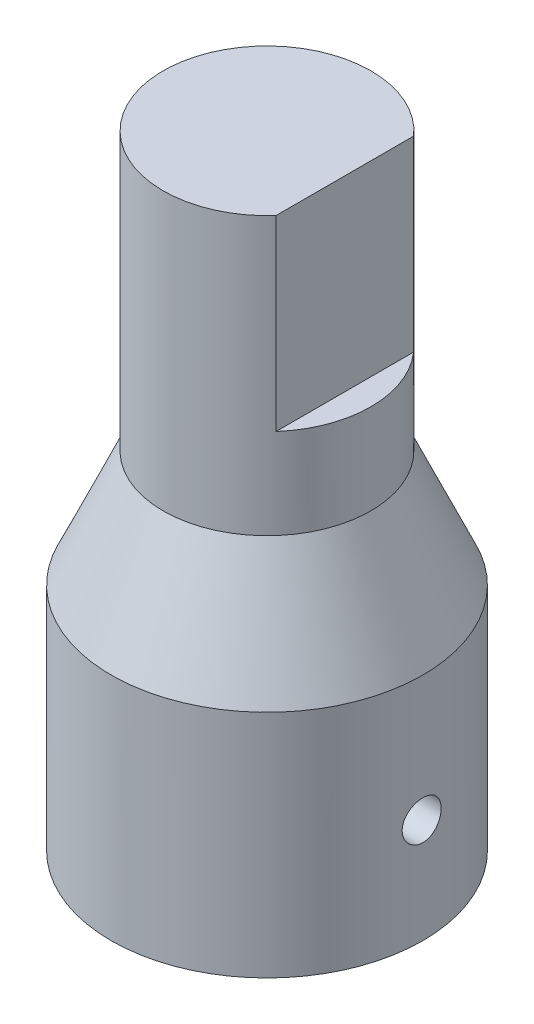
ISO-10303-21;
HEADER;
FILE_DESCRIPTION(('STEP AP214'),'2;1');
FILE_NAME('part.step','',(''),(''),'','','');
FILE_SCHEMA(('AUTOMOTIVE_DESIGN { 1 0 10303 214 1 1 1 1 }'));
ENDSEC;
DATA;
#1=APPLICATION_CONTEXT('core data for automotive mechanical design processes');
#2=APPLICATION_PROTOCOL_DEFINITION('international standard','automotive_design',2000,#1);
#3=PRODUCT_CONTEXT('',#1,'mechanical');
#4=PRODUCT('Part','Part','',(#3));
#5=PRODUCT_RELATED_PRODUCT_CATEGORY('part','',(#4));
#6=PRODUCT_DEFINITION_FORMATION('','',#4);
#7=PRODUCT_DEFINITION_CONTEXT('part definition',#1,'design');
#8=PRODUCT_DEFINITION('design','',#6,#7);
#9=PRODUCT_DEFINITION_SHAPE('','',#8);
#10=(LENGTH_UNIT() NAMED_UNIT(*) SI_UNIT(.MILLI.,.METRE.));
#11=(NAMED_UNIT(*) PLANE_ANGLE_UNIT() SI_UNIT($,.RADIAN.));
#12=(NAMED_UNIT(*) SI_UNIT($,.STERADIAN.) SOLID_ANGLE_UNIT());
#13=UNCERTAINTY_MEASURE_WITH_UNIT(LENGTH_MEASURE(1.E-05),#10,'distance_accuracy_value','');
#14=(GEOMETRIC_REPRESENTATION_CONTEXT(3) GLOBAL_UNCERTAINTY_ASSIGNED_CONTEXT((#13)) GLOBAL_UNIT_ASSIGNED_CONTEXT((#10,
#11,#12)) REPRESENTATION_CONTEXT('',''));
#15=CARTESIAN_POINT('',(0.,0.,0.));
#16=DIRECTION('',(0.,0.,1.));
#17=DIRECTION('',(1.,0.,0.));
#18=AXIS2_PLACEMENT_3D('',#15,#16,#17);
#19=CARTESIAN_POINT('',(0.,14.06,0.));
#20=DIRECTION('',(0.,-1.,0.));
#21=DIRECTION('',(0.,0.,-1.));
#22=AXIS2_PLACEMENT_3D('',#19,#20,#21);
#23=CYLINDRICAL_SURFACE('',#22,9.525);
#24=CARTESIAN_POINT('',(0.,14.06,0.));
#25=DIRECTION('',(0.,-1.,0.));
#26=DIRECTION('',(0.,0.,-1.));
#27=AXIS2_PLACEMENT_3D('',#24,#25,#26);
#28=CIRCLE('',#27,9.525);
#29=CARTESIAN_POINT('',(0.,14.06,-9.525));
#30=VERTEX_POINT('',#29);
#31=EDGE_CURVE('E79',#30,#30,#28,.F.);
#32=ORIENTED_EDGE('',*,*,#31,.F.);
#33=EDGE_LOOP('',(#32));
#34=FACE_BOUND('',#33,.T.);
#35=CARTESIAN_POINT('',(0.,0.,0.));
#36=DIRECTION('',(0.,1.,0.));
#37=DIRECTION('',(0.,0.,1.));
#38=AXIS2_PLACEMENT_3D('',#35,#36,#37);
#39=CIRCLE('',#38,9.525);
#40=CARTESIAN_POINT('',(0.,0.,9.525));
#41=VERTEX_POINT('',#40);
#42=EDGE_CURVE('E91',#41,#41,#39,.T.);
#43=ORIENTED_EDGE('',*,*,#42,.T.);
#44=EDGE_LOOP('',(#43));
#45=FACE_BOUND('',#44,.T.);
#46=CARTESIAN_POINT('',(9.45037168581215,6.38,1.19));
#47=CARTESIAN_POINT('',(9.45037264153151,6.31343763360096,1.18999716991653));
#48=CARTESIAN_POINT('',(9.45108251308956,6.24683365884784,1.1843964303129));
#49=CARTESIAN_POINT('',(9.45384422599999,6.11547928977974,1.16214251532668));
#50=CARTESIAN_POINT('',(9.45589746984964,6.05073090654836,1.14547778873659));
#51=CARTESIAN_POINT('',(9.46110981514661,5.92500853678741,1.10159483656561));
#52=CARTESIAN_POINT('',(9.46426816613176,5.86403202182239,1.07438377150283));
#53=CARTESIAN_POINT('',(9.47133395466148,5.7475222134488,1.01019588043544));
#54=CARTESIAN_POINT('',(9.47524126405582,5.691987991292,0.973220724703552));
#55=CARTESIAN_POINT('',(9.48338917829167,5.58761734378629,0.890332801063359));
#56=CARTESIAN_POINT('',(9.48763134988199,5.53881574535426,0.844376329040483));
#57=CARTESIAN_POINT('',(9.49595691130435,5.44959647319169,0.744924376498652));
#58=CARTESIAN_POINT('',(9.50004029323059,5.40917921646723,0.691428521220839));
#59=CARTESIAN_POINT('',(9.5076042146436,5.33775104258135,0.578197512107269));
#60=CARTESIAN_POINT('',(9.51108271819785,5.30677163849966,0.518442331675223));
#61=CARTESIAN_POINT('',(9.51702773167735,5.25530040739616,0.394526840092954));
#62=CARTESIAN_POINT('',(9.51949427912391,5.23480819152343,0.330366692373087));
#63=CARTESIAN_POINT('',(9.52312643380533,5.20499707510872,0.199818674007887));
#64=CARTESIAN_POINT('',(9.52429877975999,5.19562027914244,0.133444214479628));
#65=CARTESIAN_POINT('',(9.52523345022345,5.18812675008786,5.4171031885184E-05));
#66=CARTESIAN_POINT('',(9.52499583014668,5.19000957447439,-0.0669613875877963));
#67=CARTESIAN_POINT('',(9.52314279467513,5.20493543907906,-0.199337403060523));
#68=CARTESIAN_POINT('',(9.52153506646859,5.2179162139632,-0.264705003295682));
#69=CARTESIAN_POINT('',(9.51713109983186,5.2545721705004,-0.392326661691793));
#70=CARTESIAN_POINT('',(9.5143348388273,5.27824755528178,-0.454580660689544));
#71=CARTESIAN_POINT('',(9.50785476589063,5.33568689520442,-0.57440072392236));
#72=CARTESIAN_POINT('',(9.5041685883766,5.36947779791912,-0.631953736900307));
#73=CARTESIAN_POINT('',(9.49632108787332,5.44616937011639,-0.740595739392311));
#74=CARTESIAN_POINT('',(9.49215974311959,5.48907045695765,-0.791684432589693));
#75=CARTESIAN_POINT('',(9.4837940809287,5.58311333196171,-0.886313374417254));
#76=CARTESIAN_POINT('',(9.47958966407611,5.63430938396301,-0.929799704260077));
#77=CARTESIAN_POINT('',(9.47163976542179,5.74330250640203,-1.00757044992837));
#78=CARTESIAN_POINT('',(9.46789428505592,5.80109959749108,-1.04185483696445));
#79=CARTESIAN_POINT('',(9.461286366945,5.92170218000654,-1.10025156744196));
#80=CARTESIAN_POINT('',(9.45842430411225,5.98450978364658,-1.12435959374305));
#81=CARTESIAN_POINT('',(9.45391457914727,6.11332556338726,-1.16167145862918));
#82=CARTESIAN_POINT('',(9.45226685855337,6.17933358524813,-1.17487582214934));
#83=CARTESIAN_POINT('',(9.4503830576482,6.31220027581877,-1.18993413525669));
#84=CARTESIAN_POINT('',(9.45013754054481,6.37905021610411,-1.19186396418473));
#85=CARTESIAN_POINT('',(9.45106098640868,6.51212045912965,-1.18451863421254));
#86=CARTESIAN_POINT('',(9.45222991925946,6.57834077524554,-1.17524371388379));
#87=CARTESIAN_POINT('',(9.45584194377805,6.70804463948868,-1.14581605336035));
#88=CARTESIAN_POINT('',(9.45828073101195,6.77153665354108,-1.125700053228));
#89=CARTESIAN_POINT('',(9.46415418223574,6.89424645557599,-1.07519907196292));
#90=CARTESIAN_POINT('',(9.46758888117965,6.95346409344744,-1.04481373039573));
#91=CARTESIAN_POINT('',(9.47508975436793,7.06628748014224,-0.974450020430184));
#92=CARTESIAN_POINT('',(9.47915916429753,7.1198619761186,-0.934421890790981));
#93=CARTESIAN_POINT('',(9.48746077568779,7.21955941966134,-0.845979202945391));
#94=CARTESIAN_POINT('',(9.49169298346884,7.26568207755892,-0.797564318879548));
#95=CARTESIAN_POINT('',(9.4998723107226,7.34943313065488,-0.693390980417168));
#96=CARTESIAN_POINT('',(9.5038176697801,7.38701166665858,-0.637592283310463));
#97=CARTESIAN_POINT('',(9.51095243606812,7.45226276847941,-0.520430956263431));
#98=CARTESIAN_POINT('',(9.51414185852176,7.4799355337856,-0.459068438402256));
#99=CARTESIAN_POINT('',(9.51939757374525,7.52450722689759,-0.332687033687352));
#100=CARTESIAN_POINT('',(9.52146686860327,7.54143497401439,-0.267678440724219));
#101=CARTESIAN_POINT('',(9.52426163977849,7.56412986511567,-0.135714153998385));
#102=CARTESIAN_POINT('',(9.52498717662689,7.56989751182084,-0.0687585480792384));
#103=CARTESIAN_POINT('',(9.52501239888289,7.57009909151163,0.0647122895703891));
#104=CARTESIAN_POINT('',(9.52432175662993,7.56460990732446,0.131227416461207));
#105=CARTESIAN_POINT('',(9.52161144912067,7.54261647241155,0.26238193590744));
#106=CARTESIAN_POINT('',(9.51959178478192,7.52611222929047,0.327021329757808));
#107=CARTESIAN_POINT('',(9.51444936789292,7.48258130341164,0.452579463158118));
#108=CARTESIAN_POINT('',(9.51132700095355,7.45555829868751,0.513499494631467));
#109=CARTESIAN_POINT('',(9.50432492428026,7.39176490093249,0.629952236022893));
#110=CARTESIAN_POINT('',(9.50044520558124,7.35499439251425,0.685484882156463));
#111=CARTESIAN_POINT('',(9.4923298874484,7.27246531130851,0.789979263186505));
#112=CARTESIAN_POINT('',(9.48809212661981,7.2266495327557,0.838895652055997));
#113=CARTESIAN_POINT('',(9.47975569136095,7.1274492229981,0.928376018315304));
#114=CARTESIAN_POINT('',(9.47565705011555,7.07406290146226,0.968938014423616));
#115=CARTESIAN_POINT('',(9.46804605795317,6.96100081172117,1.04069195281877));
#116=CARTESIAN_POINT('',(9.46453602974224,6.90130157540942,1.07184714494874));
#117=CARTESIAN_POINT('',(9.45852691404486,6.77750807150617,1.12364570369548));
#118=CARTESIAN_POINT('',(9.4560267275397,6.71341867112672,1.14430050434002));
#119=CARTESIAN_POINT('',(9.45292749587681,6.60416460922818,1.16956651409533));
#120=CARTESIAN_POINT('',(9.45197383987563,6.55968909404729,1.17721805327143));
#121=CARTESIAN_POINT('',(9.45069561356315,6.47014874568561,1.18743573539382));
#122=CARTESIAN_POINT('',(9.45037103848582,6.42508391697216,1.19000191686767));
#123=CARTESIAN_POINT('',(9.45037168581215,6.38,1.19));
#124=B_SPLINE_CURVE_WITH_KNOTS('',3,(#46,#47,#48,#49,#50,#51,#52,#53,#54,#55,#56,#57,#58,#59,
#60,#61,#62,#63,#64,#65,#66,#67,#68,#69,#70,#71,#72,#73,#74,#75,#76,#77,#78,#79,#80,#81,#82,#83,
#84,#85,#86,#87,#88,#89,#90,#91,#92,#93,#94,#95,#96,#97,#98,#99,#100,#101,#102,#103,#104,#105,
#106,#107,#108,#109,#110,#111,#112,#113,#114,#115,#116,#117,#118,#119,#120,#121,#122,#123),
.UNSPECIFIED.,.T.,.F.,(4,2,2,2,2,2,2,2,2,2,2,2,2,2,2,2,2,2,2,2,2,2,2,2,2,2,2,2,2,2,2,2,2,2,2,2,
2,2,4),(0.,0.199522399972923,0.399253436900873,0.598849101788066,0.798410645373971,
0.998968609282526,1.19953654581048,1.40076702034379,1.60199003297955,1.80216029108681,
2.00232268216225,2.20136937178266,2.40041984215972,2.60000537137378,2.79960004603763,
3.00055746048545,3.20151550364546,3.40255871421423,3.60359224539375,3.80327121734763,
4.00294593781248,4.20194818383015,4.4009574151758,4.60101649566635,4.80108335100855,
5.00228933136802,5.20349125947837,5.40415123610588,5.60480217354306,5.80408725360614,
6.00337219608515,6.20258751827357,6.40180519880469,6.6023256823584,6.80289366562246,
7.00423537300967,7.20535736435751,7.34049858531238,7.47563878241023),.UNSPECIFIED.);
#125=CARTESIAN_POINT('',(9.45037168581215,6.38,1.19));
#126=VERTEX_POINT('',#125);
#127=EDGE_CURVE('E137',#126,#126,#124,.T.);
#128=ORIENTED_EDGE('',*,*,#127,.F.);
#129=EDGE_LOOP('',(#128));
#130=FACE_BOUND('',#129,.T.);
#131=ADVANCED_FACE('F43',(#34,#45,#130),#23,.T.);
#132=CARTESIAN_POINT('',(0.,14.06,0.));
#133=DIRECTION('',(0.,-1.,0.));
#134=DIRECTION('',(0.,0.,-1.));
#135=AXIS2_PLACEMENT_3D('',#132,#133,#134);
#136=CYLINDRICAL_SURFACE('',#135,6.35);
#137=CARTESIAN_POINT('',(0.,14.06,0.));
#138=DIRECTION('',(0.,-1.,0.));
#139=DIRECTION('',(0.,0.,-1.));
#140=AXIS2_PLACEMENT_3D('',#137,#138,#139);
#141=CIRCLE('',#140,6.35);
#142=CARTESIAN_POINT('',(0.,14.06,-6.35));
#143=VERTEX_POINT('',#142);
#144=EDGE_CURVE('E144',#143,#143,#141,.T.);
#145=ORIENTED_EDGE('',*,*,#144,.F.);
#146=EDGE_LOOP('',(#145));
#147=FACE_BOUND('',#146,.T.);
#148=CARTESIAN_POINT('',(0.,0.,0.));
#149=DIRECTION('',(0.,-1.,0.));
#150=DIRECTION('',(0.,0.,-1.));
#151=AXIS2_PLACEMENT_3D('',#148,#149,#150);
#152=CIRCLE('',#151,6.35);
#153=CARTESIAN_POINT('',(0.,0.,-6.35));
#154=VERTEX_POINT('',#153);
#155=EDGE_CURVE('E142',#154,#154,#152,.T.);
#156=ORIENTED_EDGE('',*,*,#155,.T.);
#157=EDGE_LOOP('',(#156));
#158=FACE_BOUND('',#157,.T.);
#159=CARTESIAN_POINT('',(6.23749949899798,6.38,1.19));
#160=CARTESIAN_POINT('',(6.23750078026261,6.44621005322413,1.18999745972019));
#161=CARTESIAN_POINT('',(6.23856516125152,6.51245307174854,1.18445549061902));
#162=CARTESIAN_POINT('',(6.24270238343881,6.6430712585922,1.16244896292699));
#163=CARTESIAN_POINT('',(6.24577692913486,6.70744479327753,1.14597513460551));
#164=CARTESIAN_POINT('',(6.25357431695067,6.83241517642426,1.10262852836323));
#165=CARTESIAN_POINT('',(6.25829562402851,6.89301548034891,1.07576543235335));
#166=CARTESIAN_POINT('',(6.2688527438643,7.00884538232623,1.01242846911454));
#167=CARTESIAN_POINT('',(6.2746884694542,7.06407539992465,0.97595535348152));
#168=CARTESIAN_POINT('',(6.28689792642734,7.16828773759325,0.893950345694622));
#169=CARTESIAN_POINT('',(6.29327692734904,7.21719359759681,0.848322057689071));
#170=CARTESIAN_POINT('',(6.30580763864063,7.30670319626329,0.749510255370385));
#171=CARTESIAN_POINT('',(6.31195933407418,7.34730639014685,0.696326245676426));
#172=CARTESIAN_POINT('',(6.32339874913363,7.4193510367955,0.583410530974325));
#173=CARTESIAN_POINT('',(6.32867953647516,7.4507204053366,0.523632070986402));
#174=CARTESIAN_POINT('',(6.33772315208374,7.50294252845517,0.399537974600996));
#175=CARTESIAN_POINT('',(6.34148610501512,7.5237961467582,0.335222711334857));
#176=CARTESIAN_POINT('',(6.34703284970264,7.55415839406284,0.204672981861456));
#177=CARTESIAN_POINT('',(6.34883910987182,7.56379591352581,0.138469462402981));
#178=CARTESIAN_POINT('',(6.35034639387622,7.57185398879645,0.0053621812782321));
#179=CARTESIAN_POINT('',(6.35004759679846,7.57027549880209,-0.0615415203367523));
#180=CARTESIAN_POINT('',(6.34739599219528,7.55604522087716,-0.193266108981925));
#181=CARTESIAN_POINT('',(6.34506892879018,7.54353221603618,-0.258102581921304));
#182=CARTESIAN_POINT('',(6.33865113768287,7.50800759901928,-0.38473898180573));
#183=CARTESIAN_POINT('',(6.33456034575559,7.48499560452736,-0.446538798081501));
#184=CARTESIAN_POINT('',(6.32503171329325,7.42899396992299,-0.565750219062392));
#185=CARTESIAN_POINT('',(6.31958641289168,7.39594884288113,-0.623135137199623));
#186=CARTESIAN_POINT('',(6.3079509674285,7.32085985738842,-0.731597201950985));
#187=CARTESIAN_POINT('',(6.30176074672389,7.27881508472967,-0.782673706907869));
#188=CARTESIAN_POINT('',(6.28920920850321,7.18615551631969,-0.877891333959208));
#189=CARTESIAN_POINT('',(6.28284672261843,7.13541930570736,-0.921914229747355));
#190=CARTESIAN_POINT('',(6.27075839278776,7.02722155734565,-1.00084384377462));
#191=CARTESIAN_POINT('',(6.26503255813905,6.96975992140816,-1.03575042889576));
#192=CARTESIAN_POINT('',(6.25486413987407,6.84958578294708,-1.09549021666779));
#193=CARTESIAN_POINT('',(6.25042374700944,6.78686454843463,-1.12030625097985));
#194=CARTESIAN_POINT('',(6.2433625311351,6.65804095956337,-1.15901479823213));
#195=CARTESIAN_POINT('',(6.24074150218919,6.59193898878427,-1.17290854750374));
#196=CARTESIAN_POINT('',(6.23765651246904,6.45929638123639,-1.18920554320072));
#197=CARTESIAN_POINT('',(6.23716066944776,6.39277733272415,-1.19177863887631));
#198=CARTESIAN_POINT('',(6.23829687782516,6.26026005370896,-1.18581657464029));
#199=CARTESIAN_POINT('',(6.23992882410675,6.19426179763987,-1.17728196347184));
#200=CARTESIAN_POINT('',(6.24510703467551,6.06521785772552,-1.14949255723867));
#201=CARTESIAN_POINT('',(6.24863739352759,6.00215230597804,-1.13032679150002));
#202=CARTESIAN_POINT('',(6.25720094453764,5.88012761734596,-1.08191358131688));
#203=CARTESIAN_POINT('',(6.26223424735253,5.82116878322011,-1.05266539451161));
#204=CARTESIAN_POINT('',(6.27330916940283,5.7082828543774,-0.984526619256281));
#205=CARTESIAN_POINT('',(6.27936174687189,5.65442162423767,-0.945528727348812));
#206=CARTESIAN_POINT('',(6.29176241291361,5.5539461255804,-0.859142256605887));
#207=CARTESIAN_POINT('',(6.2981105279895,5.5073325086472,-0.81175292417047));
#208=CARTESIAN_POINT('',(6.31048943918087,5.42204094145246,-0.709170216058338));
#209=CARTESIAN_POINT('',(6.316514868931,5.38347721693516,-0.653881118633038));
#210=CARTESIAN_POINT('',(6.32747922465622,5.31618624816834,-0.537510237310789));
#211=CARTESIAN_POINT('',(6.33241819242796,5.28745862549619,-0.476428676381761));
#212=CARTESIAN_POINT('',(6.34063005728923,5.24082635641034,-0.350522475511806));
#213=CARTESIAN_POINT('',(6.34391157822906,5.22286559572911,-0.285719205908492));
#214=CARTESIAN_POINT('',(6.34847559724797,5.19809780528843,-0.153948610563211));
#215=CARTESIAN_POINT('',(6.34975830543563,5.19128960320511,-0.086981513031147));
#216=CARTESIAN_POINT('',(6.35017600053786,5.18906096960872,0.0461203195725555));
#217=CARTESIAN_POINT('',(6.34934352630838,5.19346801033821,0.112252125580659));
#218=CARTESIAN_POINT('',(6.3456920050971,5.21316692161687,0.242815271554796));
#219=CARTESIAN_POINT('',(6.34287297711735,5.22845868804999,0.30724662778009));
#220=CARTESIAN_POINT('',(6.33556507456714,5.26942030676389,0.432488844623476));
#221=CARTESIAN_POINT('',(6.33107915298483,5.29507181317,0.493305888490748));
#222=CARTESIAN_POINT('',(6.32092309466721,5.35600408370262,0.609798425416549));
#223=CARTESIAN_POINT('',(6.3152528787102,5.39128549205617,0.665473574155821));
#224=CARTESIAN_POINT('',(6.3032515687894,5.47106999737169,0.770961663863636));
#225=CARTESIAN_POINT('',(6.29691218406044,5.51569774504503,0.820679394552785));
#226=CARTESIAN_POINT('',(6.28433937847151,5.61264944961917,0.911980157400864));
#227=CARTESIAN_POINT('',(6.2781059828841,5.66497521414173,0.953561273589892));
#228=CARTESIAN_POINT('',(6.26638797766641,5.77641607881666,1.02776945897011));
#229=CARTESIAN_POINT('',(6.26091082012314,5.8355894524784,1.06031023015317));
#230=CARTESIAN_POINT('',(6.25141509395909,5.95864671949259,1.11493693768154));
#231=CARTESIAN_POINT('',(6.24739514899,6.02252609899368,1.13703274540451));
#232=CARTESIAN_POINT('',(6.2421074557308,6.13549524949637,1.16565023261791));
#233=CARTESIAN_POINT('',(6.24038973096045,6.18392352847998,1.17476575000297));
#234=CARTESIAN_POINT('',(6.23808529163837,6.28156181125071,1.18694149580345));
#235=CARTESIAN_POINT('',(6.23749854635776,6.33077179376219,1.19000188873762));
#236=CARTESIAN_POINT('',(6.23749949899798,6.38,1.19));
#237=B_SPLINE_CURVE_WITH_KNOTS('',3,(#159,#160,#161,#162,#163,#164,#165,#166,#167,#168,#169,
#170,#171,#172,#173,#174,#175,#176,#177,#178,#179,#180,#181,#182,#183,#184,#185,#186,#187,#188,
#189,#190,#191,#192,#193,#194,#195,#196,#197,#198,#199,#200,#201,#202,#203,#204,#205,#206,#207,
#208,#209,#210,#211,#212,#213,#214,#215,#216,#217,#218,#219,#220,#221,#222,#223,#224,#225,#226,
#227,#228,#229,#230,#231,#232,#233,#234,#235,#236),.UNSPECIFIED.,.T.,.F.,(4,2,2,2,2,2,2,2,2,2,2,
2,2,2,2,2,2,2,2,2,2,2,2,2,2,2,2,2,2,2,2,2,2,2,2,2,2,2,4),(0.,0.198450008627837,
0.397068509438012,0.595502359037317,0.793920693806321,0.994549586409423,1.19519163905423,
1.39736082304709,1.59951339889127,1.79931924319469,1.99910808929113,2.1963974133463,
2.39369392217731,2.59210206693382,2.79053037608965,2.99199833761527,3.19346924084741,
3.39528151208978,3.59707093620967,3.79582226034929,3.99456376614469,4.19166552785484,
4.38878180511398,4.58817115938399,4.78757842906274,4.98964728616902,5.19170836824156,
5.3927069885915,5.59368447920657,5.79158901689205,5.98949166157949,6.18704537013806,
6.38461229800574,6.58500431890193,6.78544347049006,6.98773493790894,7.18983483857971,
7.33738952132504,7.48494019492979),.UNSPECIFIED.);
#238=CARTESIAN_POINT('',(6.23749949899798,6.38,1.19));
#239=VERTEX_POINT('',#238);
#240=EDGE_CURVE('E50',#239,#239,#237,.T.);
#241=ORIENTED_EDGE('',*,*,#240,.F.);
#242=EDGE_LOOP('',(#241));
#243=FACE_BOUND('',#242,.T.);
#244=ADVANCED_FACE('F120',(#147,#158,#243),#136,.F.);
#245=CARTESIAN_POINT('',(0.,0.,0.));
#246=DIRECTION('',(0.,1.,0.));
#247=DIRECTION('',(0.,0.,1.));
#248=AXIS2_PLACEMENT_3D('',#245,#246,#247);
#249=PLANE('',#248);
#250=ORIENTED_EDGE('',*,*,#155,.F.);
#251=EDGE_LOOP('',(#250));
#252=FACE_BOUND('',#251,.T.);
#253=ORIENTED_EDGE('',*,*,#42,.F.);
#254=EDGE_LOOP('',(#253));
#255=FACE_BOUND('',#254,.T.);
#256=ADVANCED_FACE('F113',(#252,#255),#249,.F.);
#257=CARTESIAN_POINT('',(0.,21.16,0.));
#258=DIRECTION('',(0.,-1.,0.));
#259=DIRECTION('',(0.,0.,-1.));
#260=AXIS2_PLACEMENT_3D('',#257,#258,#259);
#261=CONICAL_SURFACE('',#260,6.35,0.420508920904782);
#262=CARTESIAN_POINT('',(0.,21.16,0.));
#263=DIRECTION('',(0.,1.,0.));
#264=DIRECTION('',(0.,0.,1.));
#265=AXIS2_PLACEMENT_3D('',#262,#263,#264);
#266=CIRCLE('',#265,6.35);
#267=CARTESIAN_POINT('',(0.,21.16,6.35));
#268=VERTEX_POINT('',#267);
#269=EDGE_CURVE('E90',#268,#268,#266,.T.);
#270=ORIENTED_EDGE('',*,*,#269,.F.);
#271=EDGE_LOOP('',(#270));
#272=FACE_BOUND('',#271,.T.);
#273=ORIENTED_EDGE('',*,*,#31,.T.);
#274=EDGE_LOOP('',(#273));
#275=FACE_BOUND('',#274,.T.);
#276=ADVANCED_FACE('F104',(#272,#275),#261,.T.);
#277=CARTESIAN_POINT('',(0.,38.1,0.));
#278=DIRECTION('',(0.,-1.,0.));
#279=DIRECTION('',(0.,0.,-1.));
#280=AXIS2_PLACEMENT_3D('',#277,#278,#279);
#281=CYLINDRICAL_SURFACE('',#280,6.35);
#282=CARTESIAN_POINT('',(0.,38.1,0.));
#283=DIRECTION('',(0.,1.,0.));
#284=DIRECTION('',(0.,0.,1.));
#285=AXIS2_PLACEMENT_3D('',#282,#283,#284);
#286=CIRCLE('',#285,6.35);
#287=CARTESIAN_POINT('',(4.76,38.1,-4.20296324038172));
#288=VERTEX_POINT('',#287);
#289=CARTESIAN_POINT('',(4.76,38.1,4.20296324038172));
#290=VERTEX_POINT('',#289);
#291=EDGE_CURVE('E81',#288,#290,#286,.T.);
#292=ORIENTED_EDGE('',*,*,#291,.F.);
#293=DIRECTION('',(0.,-1.,0.));
#294=VECTOR('',#293,1.);
#295=CARTESIAN_POINT('',(4.76,38.1,-4.20296324038172));
#296=LINE('',#295,#294);
#297=CARTESIAN_POINT('',(4.76,26.67,-4.20296324038172));
#298=VERTEX_POINT('',#297);
#299=EDGE_CURVE('E61',#288,#298,#296,.T.);
#300=ORIENTED_EDGE('',*,*,#299,.T.);
#301=CARTESIAN_POINT('',(0.,26.67,0.));
#302=DIRECTION('',(0.,-1.,0.));
#303=DIRECTION('',(0.,0.,-1.));
#304=AXIS2_PLACEMENT_3D('',#301,#302,#303);
#305=CIRCLE('',#304,6.35);
#306=CARTESIAN_POINT('',(4.76,26.67,4.20296324038172));
#307=VERTEX_POINT('',#306);
#308=EDGE_CURVE('E12',#298,#307,#305,.T.);
#309=ORIENTED_EDGE('',*,*,#308,.T.);
#310=DIRECTION('',(0.,-1.,0.));
#311=VECTOR('',#310,1.);
#312=CARTESIAN_POINT('',(4.76,38.1,4.20296324038172));
#313=LINE('',#312,#311);
#314=EDGE_CURVE('E66',#307,#290,#313,.F.);
#315=ORIENTED_EDGE('',*,*,#314,.T.);
#316=EDGE_LOOP('',(#292,#300,#309,#315));
#317=FACE_BOUND('',#316,.T.);
#318=ORIENTED_EDGE('',*,*,#269,.T.);
#319=EDGE_LOOP('',(#318));
#320=FACE_BOUND('',#319,.T.);
#321=ADVANCED_FACE('F85',(#317,#320),#281,.T.);
#322=CARTESIAN_POINT('',(0.,38.1,0.));
#323=DIRECTION('',(0.,1.,0.));
#324=DIRECTION('',(0.,0.,1.));
#325=AXIS2_PLACEMENT_3D('',#322,#323,#324);
#326=PLANE('',#325);
#327=DIRECTION('',(0.,0.,1.));
#328=VECTOR('',#327,1.);
#329=CARTESIAN_POINT('',(4.76,38.1,0.));
#330=LINE('',#329,#328);
#331=EDGE_CURVE('E60',#288,#290,#330,.T.);
#332=ORIENTED_EDGE('',*,*,#331,.F.);
#333=ORIENTED_EDGE('',*,*,#291,.T.);
#334=EDGE_LOOP('',(#332,#333));
#335=FACE_BOUND('',#334,.T.);
#336=ADVANCED_FACE('F89',(#335),#326,.T.);
#337=CARTESIAN_POINT('',(6.35,26.67,-8.47));
#338=DIRECTION('',(0.,-1.,0.));
#339=DIRECTION('',(0.,0.,-1.));
#340=AXIS2_PLACEMENT_3D('',#337,#338,#339);
#341=PLANE('',#340);
#342=DIRECTION('',(0.,0.,1.));
#343=VECTOR('',#342,1.);
#344=CARTESIAN_POINT('',(4.76,26.67,-8.47));
#345=LINE('',#344,#343);
#346=EDGE_CURVE('E83',#298,#307,#345,.T.);
#347=ORIENTED_EDGE('',*,*,#346,.T.);
#348=ORIENTED_EDGE('',*,*,#308,.F.);
#349=EDGE_LOOP('',(#347,#348));
#350=FACE_BOUND('',#349,.T.);
#351=ADVANCED_FACE('F163',(#350),#341,.F.);
#352=CARTESIAN_POINT('',(4.76,38.1,-8.47));
#353=DIRECTION('',(-1.,0.,0.));
#354=DIRECTION('',(0.,-1.,0.));
#355=AXIS2_PLACEMENT_3D('',#352,#353,#354);
#356=PLANE('',#355);
#357=ORIENTED_EDGE('',*,*,#331,.T.);
#358=ORIENTED_EDGE('',*,*,#314,.F.);
#359=ORIENTED_EDGE('',*,*,#346,.F.);
#360=ORIENTED_EDGE('',*,*,#299,.F.);
#361=EDGE_LOOP('',(#357,#358,#359,#360));
#362=FACE_BOUND('',#361,.T.);
#363=ADVANCED_FACE('F74',(#362),#356,.F.);
#364=CARTESIAN_POINT('',(0.,14.06,0.));
#365=DIRECTION('',(0.,-1.,0.));
#366=DIRECTION('',(0.,0.,-1.));
#367=AXIS2_PLACEMENT_3D('',#364,#365,#366);
#368=PLANE('',#367);
#369=ORIENTED_EDGE('',*,*,#144,.T.);
#370=EDGE_LOOP('',(#369));
#371=FACE_BOUND('',#370,.T.);
#372=ADVANCED_FACE('F153',(#371),#368,.T.);
#373=CARTESIAN_POINT('',(14.06,6.38,0.));
#374=DIRECTION('',(-1.,0.,0.));
#375=DIRECTION('',(0.,0.,1.));
#376=AXIS2_PLACEMENT_3D('',#373,#374,#375);
#377=CYLINDRICAL_SURFACE('',#376,1.19);
#378=ORIENTED_EDGE('',*,*,#240,.T.);
#379=EDGE_LOOP('',(#378));
#380=FACE_BOUND('',#379,.T.);
#381=ORIENTED_EDGE('',*,*,#127,.T.);
#382=EDGE_LOOP('',(#381));
#383=FACE_BOUND('',#382,.T.);
#384=ADVANCED_FACE('F152',(#380,#383),#377,.F.);
#385=CLOSED_SHELL('',(#131,#244,#256,#276,#321,#336,#351,#363,#372,#384));
#386=MANIFOLD_SOLID_BREP('B2',#385);
#387=ADVANCED_BREP_SHAPE_REPRESENTATION('',(#18,#386),#14);
#388=SHAPE_DEFINITION_REPRESENTATION(#9,#387);
ENDSEC;
END-ISO-10303-21;
